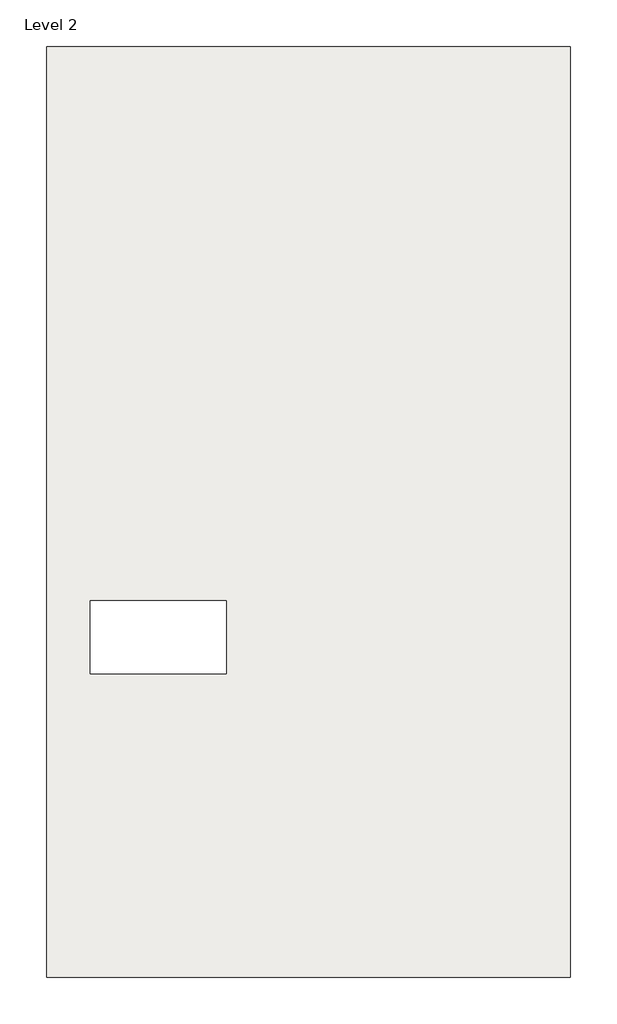
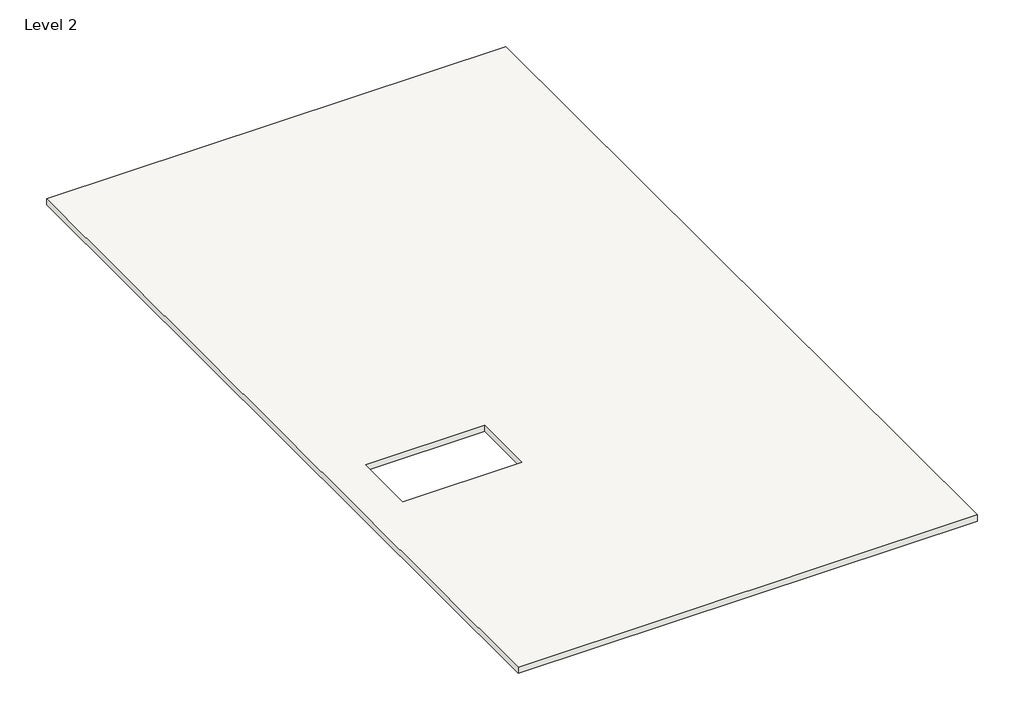
# One storey, incomplete: 1 roof.
"""IFC4 building model written with IfcOpenShell, lengths in millimetres."""

from ifc_helpers import new_model, si_unit, frame, origin, place, context, project, spatial, polyline, outline, extrude, element, save

model = new_model("IFC4")

# Units and contexts
model_context = context("Model", 3, world=origin())
ifc_project = project(units=[si_unit("LENGTHUNIT", "METRE", prefix="MILLI")], contexts=[model_context])

# Site, building, storey
site = spatial("IfcSite", under=ifc_project)
building = spatial("IfcBuilding", under=site)
storey = spatial("IfcBuildingStorey", under=building, Name="Level 2", Elevation=3048.0)

# Roof
placement = place(None, origin())
element("IfcRoof", 1, ObjectType="ROOF 6\"", at=placement, inside=storey, context=model_context, shape_type="SweptSolid", body=[
    extrude(outline(polyline([(4193.9879845, 9374.2934309), (4193.9879845, -9993.2065691), (-6702.6120155, -9993.2065691), (-6702.6120155, 9374.2934309), (4193.9879845, 9374.2934309)]), holes=[polyline([(-2968.8120155, -2150.9565691), (-5788.2120155, -2150.9565691), (-5788.2120155, -3674.9565691), (-2968.8120155, -3674.9565691), (-2968.8120155, -2150.9565691)])]), frame((0.0, 0.0, 3048.0), z_axis=(0.0, 0.0, 1.0), x_axis=(1.0, 0.0, 0.0)), (0.0, 0.0, 1.0), 152.4),
])

save(model, "model.ifc")

# Revit data of these elements
# Type "ROOF 6\""
#   Assembly Code = "B1020"
#   Layers, outside or top first: 0' - 6" no material (function 1)
# Element 1 (IfcRoof, "ROOF 6\"")
#   built-in parameter 1001705 = 10.5 (stored number, unit not read)
#   built-in parameter 1001710 = 33615
#   Phase Created = New Construction
#   Materials on its faces: "Default Roof", "Brick, Common", "Birch"
# Materials
#   "Default Roof": colour RGB 88 101 114, transparency 0, Cost = 0
#   "Brick, Common": class "Masonry", colour RGB 170 98 104, transparency 0, Description = "Common brick", Cost = 0
#   "Birch": class "Wood", colour RGB 224 178 126, transparency 0, Description = "Betula Alleghaniensis", Cost = 0
